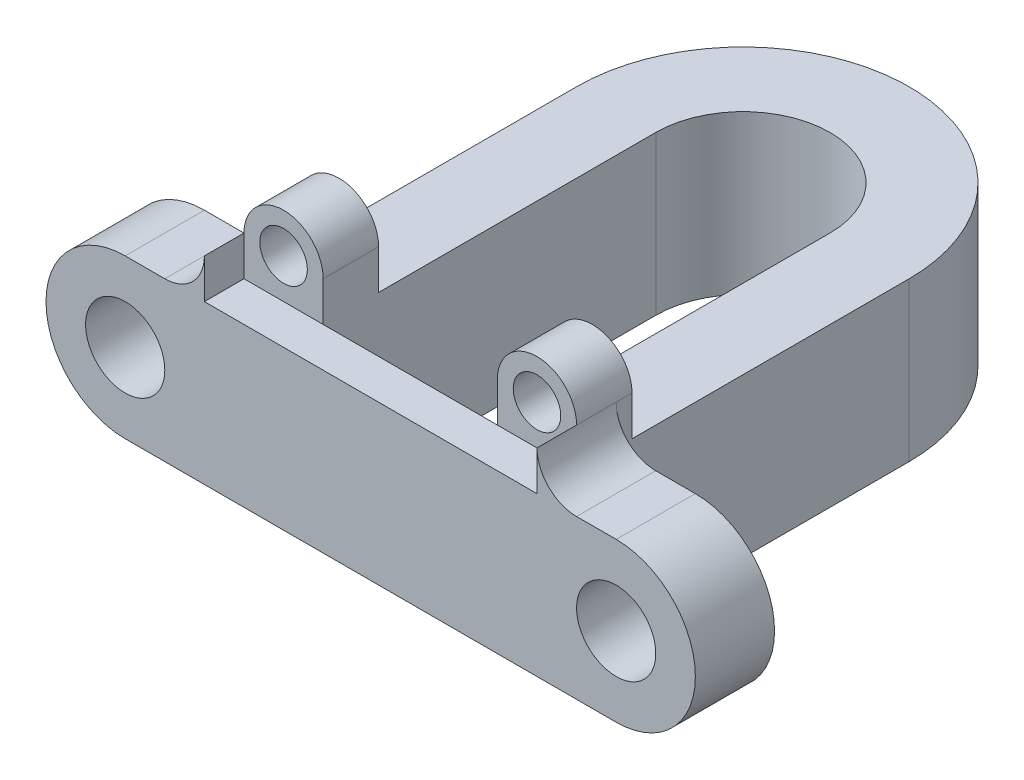
ISO-10303-21;
HEADER;
FILE_DESCRIPTION(('STEP AP214'),'2;1');
FILE_NAME('part.step','',(''),(''),'','','');
FILE_SCHEMA(('AUTOMOTIVE_DESIGN { 1 0 10303 214 1 1 1 1 }'));
ENDSEC;
DATA;
#1=APPLICATION_CONTEXT('core data for automotive mechanical design processes');
#2=APPLICATION_PROTOCOL_DEFINITION('international standard','automotive_design',2000,#1);
#3=PRODUCT_CONTEXT('',#1,'mechanical');
#4=PRODUCT('Part','Part','',(#3));
#5=PRODUCT_RELATED_PRODUCT_CATEGORY('part','',(#4));
#6=PRODUCT_DEFINITION_FORMATION('','',#4);
#7=PRODUCT_DEFINITION_CONTEXT('part definition',#1,'design');
#8=PRODUCT_DEFINITION('design','',#6,#7);
#9=PRODUCT_DEFINITION_SHAPE('','',#8);
#10=(LENGTH_UNIT() NAMED_UNIT(*) SI_UNIT(.MILLI.,.METRE.));
#11=(NAMED_UNIT(*) PLANE_ANGLE_UNIT() SI_UNIT($,.RADIAN.));
#12=(NAMED_UNIT(*) SI_UNIT($,.STERADIAN.) SOLID_ANGLE_UNIT());
#13=UNCERTAINTY_MEASURE_WITH_UNIT(LENGTH_MEASURE(1.E-05),#10,'distance_accuracy_value','');
#14=(GEOMETRIC_REPRESENTATION_CONTEXT(3) GLOBAL_UNCERTAINTY_ASSIGNED_CONTEXT((#13)) GLOBAL_UNIT_ASSIGNED_CONTEXT((#10,
#11,#12)) REPRESENTATION_CONTEXT('',''));
#15=CARTESIAN_POINT('',(0.,0.,0.));
#16=DIRECTION('',(0.,0.,1.));
#17=DIRECTION('',(1.,0.,0.));
#18=AXIS2_PLACEMENT_3D('',#15,#16,#17);
#19=CARTESIAN_POINT('',(42.,0.,5.));
#20=DIRECTION('',(-1.,0.,0.));
#21=DIRECTION('',(0.,0.,1.));
#22=AXIS2_PLACEMENT_3D('',#19,#20,#21);
#23=PLANE('',#22);
#24=DIRECTION('',(0.,1.,0.));
#25=VECTOR('',#24,1.);
#26=CARTESIAN_POINT('',(42.,20.,-5.));
#27=LINE('',#26,#25);
#28=CARTESIAN_POINT('',(42.,0.,-5.));
#29=VERTEX_POINT('',#28);
#30=CARTESIAN_POINT('',(42.,25.,-5.));
#31=VERTEX_POINT('',#30);
#32=EDGE_CURVE('E53',#29,#31,#27,.T.);
#33=ORIENTED_EDGE('',*,*,#32,.F.);
#34=DIRECTION('',(0.,0.,-1.));
#35=VECTOR('',#34,1.);
#36=CARTESIAN_POINT('',(42.,0.,5.));
#37=LINE('',#36,#35);
#38=CARTESIAN_POINT('',(42.,0.,-42.));
#39=VERTEX_POINT('',#38);
#40=EDGE_CURVE('E50',#29,#39,#37,.T.);
#41=ORIENTED_EDGE('',*,*,#40,.T.);
#42=DIRECTION('',(0.,1.,0.));
#43=VECTOR('',#42,1.);
#44=CARTESIAN_POINT('',(42.,0.,-42.));
#45=LINE('',#44,#43);
#46=CARTESIAN_POINT('',(42.,20.,-42.));
#47=VERTEX_POINT('',#46);
#48=EDGE_CURVE('E386',#39,#47,#45,.T.);
#49=ORIENTED_EDGE('',*,*,#48,.T.);
#50=DIRECTION('',(0.,0.,-1.));
#51=VECTOR('',#50,1.);
#52=CARTESIAN_POINT('',(42.,20.,5.));
#53=LINE('',#52,#51);
#54=CARTESIAN_POINT('',(42.,20.,-7.));
#55=VERTEX_POINT('',#54);
#56=EDGE_CURVE('E398',#55,#47,#53,.T.);
#57=ORIENTED_EDGE('',*,*,#56,.F.);
#58=DIRECTION('',(0.,-1.,0.));
#59=VECTOR('',#58,1.);
#60=CARTESIAN_POINT('',(42.,25.,-7.));
#61=LINE('',#60,#59);
#62=CARTESIAN_POINT('',(42.,25.,-7.));
#63=VERTEX_POINT('',#62);
#64=EDGE_CURVE('E291',#63,#55,#61,.T.);
#65=ORIENTED_EDGE('',*,*,#64,.F.);
#66=DIRECTION('',(0.,0.,1.));
#67=VECTOR('',#66,1.);
#68=CARTESIAN_POINT('',(42.,25.,-7.));
#69=LINE('',#68,#67);
#70=EDGE_CURVE('E315',#63,#31,#69,.T.);
#71=ORIENTED_EDGE('',*,*,#70,.T.);
#72=EDGE_LOOP('',(#33,#41,#49,#57,#65,#71));
#73=FACE_BOUND('',#72,.T.);
#74=ADVANCED_FACE('F39',(#73),#23,.F.);
#75=CARTESIAN_POINT('',(0.,20.,5.));
#76=DIRECTION('',(1.,0.,0.));
#77=DIRECTION('',(0.,0.,-1.));
#78=AXIS2_PLACEMENT_3D('',#75,#76,#77);
#79=PLANE('',#78);
#80=DIRECTION('',(0.,1.,0.));
#81=VECTOR('',#80,1.);
#82=CARTESIAN_POINT('',(0.,25.,-5.));
#83=LINE('',#82,#81);
#84=CARTESIAN_POINT('',(0.,0.,-5.));
#85=VERTEX_POINT('',#84);
#86=CARTESIAN_POINT('',(0.,25.,-5.));
#87=VERTEX_POINT('',#86);
#88=EDGE_CURVE('E267',#85,#87,#83,.T.);
#89=ORIENTED_EDGE('',*,*,#88,.T.);
#90=DIRECTION('',(0.,0.,1.));
#91=VECTOR('',#90,1.);
#92=CARTESIAN_POINT('',(0.,25.,-7.));
#93=LINE('',#92,#91);
#94=CARTESIAN_POINT('',(0.,25.,-7.));
#95=VERTEX_POINT('',#94);
#96=EDGE_CURVE('E341',#95,#87,#93,.T.);
#97=ORIENTED_EDGE('',*,*,#96,.F.);
#98=DIRECTION('',(0.,-1.,0.));
#99=VECTOR('',#98,1.);
#100=CARTESIAN_POINT('',(0.,25.,-7.));
#101=LINE('',#100,#99);
#102=CARTESIAN_POINT('',(0.,20.,-7.));
#103=VERTEX_POINT('',#102);
#104=EDGE_CURVE('E329',#95,#103,#101,.T.);
#105=ORIENTED_EDGE('',*,*,#104,.T.);
#106=DIRECTION('',(0.,0.,-1.));
#107=VECTOR('',#106,1.);
#108=CARTESIAN_POINT('',(0.,20.,5.));
#109=LINE('',#108,#107);
#110=CARTESIAN_POINT('',(0.,20.,-42.));
#111=VERTEX_POINT('',#110);
#112=EDGE_CURVE('E399',#103,#111,#109,.T.);
#113=ORIENTED_EDGE('',*,*,#112,.T.);
#114=DIRECTION('',(0.,1.,0.));
#115=VECTOR('',#114,1.);
#116=CARTESIAN_POINT('',(0.,0.,-42.));
#117=LINE('',#116,#115);
#118=CARTESIAN_POINT('',(0.,0.,-42.));
#119=VERTEX_POINT('',#118);
#120=EDGE_CURVE('E387',#119,#111,#117,.T.);
#121=ORIENTED_EDGE('',*,*,#120,.F.);
#122=DIRECTION('',(0.,0.,-1.));
#123=VECTOR('',#122,1.);
#124=CARTESIAN_POINT('',(0.,0.,5.));
#125=LINE('',#124,#123);
#126=EDGE_CURVE('E11',#85,#119,#125,.T.);
#127=ORIENTED_EDGE('',*,*,#126,.F.);
#128=EDGE_LOOP('',(#89,#97,#105,#113,#121,#127));
#129=FACE_BOUND('',#128,.T.);
#130=ADVANCED_FACE('F41',(#129),#79,.F.);
#131=CARTESIAN_POINT('',(42.,20.,5.));
#132=DIRECTION('',(0.,-1.,0.));
#133=DIRECTION('',(0.,0.,-1.));
#134=AXIS2_PLACEMENT_3D('',#131,#132,#133);
#135=PLANE('',#134);
#136=DIRECTION('',(-1.,0.,0.));
#137=VECTOR('',#136,1.);
#138=CARTESIAN_POINT('',(42.,20.,-7.));
#139=LINE('',#138,#137);
#140=CARTESIAN_POINT('',(32.,20.,-7.));
#141=VERTEX_POINT('',#140);
#142=EDGE_CURVE('E293',#55,#141,#139,.T.);
#143=ORIENTED_EDGE('',*,*,#142,.F.);
#144=ORIENTED_EDGE('',*,*,#56,.T.);
#145=CARTESIAN_POINT('',(21.,20.,-42.));
#146=DIRECTION('',(0.,1.,0.));
#147=DIRECTION('',(0.,0.,1.));
#148=AXIS2_PLACEMENT_3D('',#145,#146,#147);
#149=CIRCLE('',#148,21.);
#150=EDGE_CURVE('E372',#47,#111,#149,.T.);
#151=ORIENTED_EDGE('',*,*,#150,.T.);
#152=ORIENTED_EDGE('',*,*,#112,.F.);
#153=DIRECTION('',(1.,0.,0.));
#154=VECTOR('',#153,1.);
#155=CARTESIAN_POINT('',(0.,20.,-7.));
#156=LINE('',#155,#154);
#157=CARTESIAN_POINT('',(10.,20.,-7.00000000000001));
#158=VERTEX_POINT('',#157);
#159=EDGE_CURVE('E318',#103,#158,#156,.T.);
#160=ORIENTED_EDGE('',*,*,#159,.T.);
#161=DIRECTION('',(0.,0.,1.));
#162=VECTOR('',#161,1.);
#163=CARTESIAN_POINT('',(10.,20.,-42.));
#164=LINE('',#163,#162);
#165=CARTESIAN_POINT('',(10.,20.,-42.));
#166=VERTEX_POINT('',#165);
#167=EDGE_CURVE('E364',#166,#158,#164,.T.);
#168=ORIENTED_EDGE('',*,*,#167,.F.);
#169=CARTESIAN_POINT('',(21.,20.,-42.));
#170=DIRECTION('',(0.,1.,0.));
#171=DIRECTION('',(0.,0.,1.));
#172=AXIS2_PLACEMENT_3D('',#169,#170,#171);
#173=CIRCLE('',#172,11.);
#174=CARTESIAN_POINT('',(32.,20.,-42.));
#175=VERTEX_POINT('',#174);
#176=EDGE_CURVE('E350',#175,#166,#173,.T.);
#177=ORIENTED_EDGE('',*,*,#176,.F.);
#178=DIRECTION('',(0.,0.,-1.));
#179=VECTOR('',#178,1.);
#180=CARTESIAN_POINT('',(32.,20.,0.));
#181=LINE('',#180,#179);
#182=EDGE_CURVE('E355',#141,#175,#181,.T.);
#183=ORIENTED_EDGE('',*,*,#182,.F.);
#184=EDGE_LOOP('',(#143,#144,#151,#152,#160,#168,#177,#183));
#185=FACE_BOUND('',#184,.T.);
#186=ADVANCED_FACE('F420',(#185),#135,.F.);
#187=CARTESIAN_POINT('',(42.,20.,5.));
#188=VERTEX_POINT('',#187);
#189=CARTESIAN_POINT('',(42.,20.,0.));
#190=VERTEX_POINT('',#189);
#191=EDGE_CURVE('E402',#188,#190,#53,.T.);
#192=ORIENTED_EDGE('',*,*,#191,.T.);
#193=DIRECTION('',(-1.,0.,0.));
#194=VECTOR('',#193,1.);
#195=CARTESIAN_POINT('',(42.,20.,0.));
#196=LINE('',#195,#194);
#197=CARTESIAN_POINT('',(32.,20.,0.));
#198=VERTEX_POINT('',#197);
#199=EDGE_CURVE('E290',#190,#198,#196,.T.);
#200=ORIENTED_EDGE('',*,*,#199,.T.);
#201=DIRECTION('',(1.,0.,0.));
#202=VECTOR('',#201,1.);
#203=CARTESIAN_POINT('',(10.,20.,0.));
#204=LINE('',#203,#202);
#205=CARTESIAN_POINT('',(10.,20.,0.));
#206=VERTEX_POINT('',#205);
#207=EDGE_CURVE('E370',#206,#198,#204,.T.);
#208=ORIENTED_EDGE('',*,*,#207,.F.);
#209=DIRECTION('',(1.,0.,0.));
#210=VECTOR('',#209,1.);
#211=CARTESIAN_POINT('',(0.,20.,0.));
#212=LINE('',#211,#210);
#213=CARTESIAN_POINT('',(0.,20.,0.));
#214=VERTEX_POINT('',#213);
#215=EDGE_CURVE('E320',#214,#206,#212,.T.);
#216=ORIENTED_EDGE('',*,*,#215,.F.);
#217=CARTESIAN_POINT('',(0.,20.,5.));
#218=VERTEX_POINT('',#217);
#219=EDGE_CURVE('E400',#218,#214,#109,.T.);
#220=ORIENTED_EDGE('',*,*,#219,.F.);
#221=DIRECTION('',(-1.,0.,0.));
#222=VECTOR('',#221,1.);
#223=CARTESIAN_POINT('',(42.,20.,5.));
#224=LINE('',#223,#222);
#225=EDGE_CURVE('E394',#188,#218,#224,.T.);
#226=ORIENTED_EDGE('',*,*,#225,.F.);
#227=EDGE_LOOP('',(#192,#200,#208,#216,#220,#226));
#228=FACE_BOUND('',#227,.T.);
#229=ADVANCED_FACE('F455',(#228),#135,.F.);
#230=CARTESIAN_POINT('',(0.,0.,5.));
#231=DIRECTION('',(0.,1.,0.));
#232=DIRECTION('',(0.,0.,1.));
#233=AXIS2_PLACEMENT_3D('',#230,#231,#232);
#234=PLANE('',#233);
#235=DIRECTION('',(0.,0.,-1.));
#236=VECTOR('',#235,1.);
#237=CARTESIAN_POINT('',(32.,0.,0.));
#238=LINE('',#237,#236);
#239=CARTESIAN_POINT('',(32.,0.,0.));
#240=VERTEX_POINT('',#239);
#241=CARTESIAN_POINT('',(32.,0.,-42.));
#242=VERTEX_POINT('',#241);
#243=EDGE_CURVE('E360',#240,#242,#238,.T.);
#244=ORIENTED_EDGE('',*,*,#243,.T.);
#245=CARTESIAN_POINT('',(21.,0.,-42.));
#246=DIRECTION('',(0.,1.,0.));
#247=DIRECTION('',(0.,0.,1.));
#248=AXIS2_PLACEMENT_3D('',#245,#246,#247);
#249=CIRCLE('',#248,11.);
#250=CARTESIAN_POINT('',(10.,0.,-42.));
#251=VERTEX_POINT('',#250);
#252=EDGE_CURVE('E347',#242,#251,#249,.T.);
#253=ORIENTED_EDGE('',*,*,#252,.T.);
#254=DIRECTION('',(0.,0.,1.));
#255=VECTOR('',#254,1.);
#256=CARTESIAN_POINT('',(10.,0.,-42.));
#257=LINE('',#256,#255);
#258=CARTESIAN_POINT('',(10.,0.,0.));
#259=VERTEX_POINT('',#258);
#260=EDGE_CURVE('E354',#251,#259,#257,.T.);
#261=ORIENTED_EDGE('',*,*,#260,.T.);
#262=DIRECTION('',(1.,0.,0.));
#263=VECTOR('',#262,1.);
#264=CARTESIAN_POINT('',(10.,0.,0.));
#265=LINE('',#264,#263);
#266=EDGE_CURVE('E358',#259,#240,#265,.T.);
#267=ORIENTED_EDGE('',*,*,#266,.T.);
#268=EDGE_LOOP('',(#244,#253,#261,#267));
#269=FACE_BOUND('',#268,.T.);
#270=DIRECTION('',(1.,0.,0.));
#271=VECTOR('',#270,1.);
#272=CARTESIAN_POINT('',(0.,0.,5.));
#273=LINE('',#272,#271);
#274=CARTESIAN_POINT('',(-10.,0.,5.));
#275=VERTEX_POINT('',#274);
#276=CARTESIAN_POINT('',(52.,0.,5.));
#277=VERTEX_POINT('',#276);
#278=EDGE_CURVE('E220',#275,#277,#273,.T.);
#279=ORIENTED_EDGE('',*,*,#278,.F.);
#280=DIRECTION('',(0.,0.,-1.));
#281=VECTOR('',#280,1.);
#282=CARTESIAN_POINT('',(-10.,0.,5.));
#283=LINE('',#282,#281);
#284=CARTESIAN_POINT('',(-10.,0.,-5.));
#285=VERTEX_POINT('',#284);
#286=EDGE_CURVE('E283',#275,#285,#283,.T.);
#287=ORIENTED_EDGE('',*,*,#286,.T.);
#288=DIRECTION('',(1.,0.,0.));
#289=VECTOR('',#288,1.);
#290=CARTESIAN_POINT('',(0.,0.,-5.));
#291=LINE('',#290,#289);
#292=EDGE_CURVE('E261',#285,#85,#291,.T.);
#293=ORIENTED_EDGE('',*,*,#292,.T.);
#294=ORIENTED_EDGE('',*,*,#126,.T.);
#295=CARTESIAN_POINT('',(21.,0.,-42.));
#296=DIRECTION('',(0.,1.,0.));
#297=DIRECTION('',(0.,0.,1.));
#298=AXIS2_PLACEMENT_3D('',#295,#296,#297);
#299=CIRCLE('',#298,21.);
#300=EDGE_CURVE('E384',#39,#119,#299,.T.);
#301=ORIENTED_EDGE('',*,*,#300,.F.);
#302=ORIENTED_EDGE('',*,*,#40,.F.);
#303=DIRECTION('',(-1.,0.,0.));
#304=VECTOR('',#303,1.);
#305=CARTESIAN_POINT('',(42.,0.,-5.));
#306=LINE('',#305,#304);
#307=CARTESIAN_POINT('',(52.,0.,-5.));
#308=VERTEX_POINT('',#307);
#309=EDGE_CURVE('E217',#308,#29,#306,.T.);
#310=ORIENTED_EDGE('',*,*,#309,.F.);
#311=DIRECTION('',(0.,0.,-1.));
#312=VECTOR('',#311,1.);
#313=CARTESIAN_POINT('',(52.,0.,5.));
#314=LINE('',#313,#312);
#315=EDGE_CURVE('E230',#277,#308,#314,.T.);
#316=ORIENTED_EDGE('',*,*,#315,.F.);
#317=EDGE_LOOP('',(#279,#287,#293,#294,#301,#302,#310,#316));
#318=FACE_BOUND('',#317,.T.);
#319=ADVANCED_FACE('F413',(#269,#318),#234,.F.);
#320=CARTESIAN_POINT('',(0.,0.,5.));
#321=DIRECTION('',(0.,0.,1.));
#322=DIRECTION('',(1.,0.,0.));
#323=AXIS2_PLACEMENT_3D('',#320,#321,#322);
#324=PLANE('',#323);
#325=ORIENTED_EDGE('',*,*,#225,.T.);
#326=DIRECTION('',(0.,1.,0.));
#327=VECTOR('',#326,1.);
#328=CARTESIAN_POINT('',(0.,20.,5.));
#329=LINE('',#328,#327);
#330=CARTESIAN_POINT('',(0.,25.,5.));
#331=VERTEX_POINT('',#330);
#332=EDGE_CURVE('E254',#218,#331,#329,.T.);
#333=ORIENTED_EDGE('',*,*,#332,.T.);
#334=CARTESIAN_POINT('',(-5.,25.,5.));
#335=DIRECTION('',(0.,0.,-1.));
#336=DIRECTION('',(1.,0.,0.));
#337=AXIS2_PLACEMENT_3D('',#334,#335,#336);
#338=CIRCLE('',#337,5.00000000000001);
#339=CARTESIAN_POINT('',(-5.,20.,5.));
#340=VERTEX_POINT('',#339);
#341=EDGE_CURVE('E257',#331,#340,#338,.T.);
#342=ORIENTED_EDGE('',*,*,#341,.T.);
#343=DIRECTION('',(-1.,0.,0.));
#344=VECTOR('',#343,1.);
#345=CARTESIAN_POINT('',(-10.,20.,5.));
#346=LINE('',#345,#344);
#347=CARTESIAN_POINT('',(-10.,20.,5.));
#348=VERTEX_POINT('',#347);
#349=EDGE_CURVE('E259',#340,#348,#346,.T.);
#350=ORIENTED_EDGE('',*,*,#349,.T.);
#351=CARTESIAN_POINT('',(-10.,10.,5.));
#352=DIRECTION('',(0.,0.,1.));
#353=DIRECTION('',(1.,0.,0.));
#354=AXIS2_PLACEMENT_3D('',#351,#352,#353);
#355=CIRCLE('',#354,10.);
#356=EDGE_CURVE('E252',#348,#275,#355,.T.);
#357=ORIENTED_EDGE('',*,*,#356,.T.);
#358=ORIENTED_EDGE('',*,*,#278,.T.);
#359=CARTESIAN_POINT('',(52.,10.,5.));
#360=DIRECTION('',(0.,0.,-1.));
#361=DIRECTION('',(-1.,0.,0.));
#362=AXIS2_PLACEMENT_3D('',#359,#360,#361);
#363=CIRCLE('',#362,10.);
#364=CARTESIAN_POINT('',(52.,20.,5.));
#365=VERTEX_POINT('',#364);
#366=EDGE_CURVE('E196',#365,#277,#363,.T.);
#367=ORIENTED_EDGE('',*,*,#366,.F.);
#368=DIRECTION('',(1.,0.,0.));
#369=VECTOR('',#368,1.);
#370=CARTESIAN_POINT('',(52.,20.,5.));
#371=LINE('',#370,#369);
#372=CARTESIAN_POINT('',(47.,20.,5.));
#373=VERTEX_POINT('',#372);
#374=EDGE_CURVE('E211',#373,#365,#371,.T.);
#375=ORIENTED_EDGE('',*,*,#374,.F.);
#376=CARTESIAN_POINT('',(47.,25.,5.));
#377=DIRECTION('',(0.,0.,1.));
#378=DIRECTION('',(-1.,0.,0.));
#379=AXIS2_PLACEMENT_3D('',#376,#377,#378);
#380=CIRCLE('',#379,5.00000000000001);
#381=CARTESIAN_POINT('',(42.,25.,5.));
#382=VERTEX_POINT('',#381);
#383=EDGE_CURVE('E224',#382,#373,#380,.T.);
#384=ORIENTED_EDGE('',*,*,#383,.F.);
#385=DIRECTION('',(0.,1.,0.));
#386=VECTOR('',#385,1.);
#387=CARTESIAN_POINT('',(42.,25.,5.));
#388=LINE('',#387,#386);
#389=EDGE_CURVE('E221',#188,#382,#388,.T.);
#390=ORIENTED_EDGE('',*,*,#389,.F.);
#391=EDGE_LOOP('',(#325,#333,#342,#350,#357,#358,#367,#375,#384,#390));
#392=FACE_BOUND('',#391,.T.);
#393=CARTESIAN_POINT('',(-10.,10.,5.));
#394=DIRECTION('',(0.,0.,1.));
#395=DIRECTION('',(1.,0.,0.));
#396=AXIS2_PLACEMENT_3D('',#393,#394,#395);
#397=CIRCLE('',#396,5.);
#398=CARTESIAN_POINT('',(-5.,10.,5.));
#399=VERTEX_POINT('',#398);
#400=EDGE_CURVE('E244',#399,#399,#397,.T.);
#401=ORIENTED_EDGE('',*,*,#400,.F.);
#402=EDGE_LOOP('',(#401));
#403=FACE_BOUND('',#402,.T.);
#404=CARTESIAN_POINT('',(52.,10.,5.));
#405=DIRECTION('',(0.,0.,-1.));
#406=DIRECTION('',(-1.,0.,0.));
#407=AXIS2_PLACEMENT_3D('',#404,#405,#406);
#408=CIRCLE('',#407,5.);
#409=CARTESIAN_POINT('',(47.,10.,5.));
#410=VERTEX_POINT('',#409);
#411=EDGE_CURVE('E235',#410,#410,#408,.T.);
#412=ORIENTED_EDGE('',*,*,#411,.T.);
#413=EDGE_LOOP('',(#412));
#414=FACE_BOUND('',#413,.T.);
#415=ADVANCED_FACE('F212',(#392,#403,#414),#324,.T.);
#416=CARTESIAN_POINT('',(21.,0.,-42.));
#417=DIRECTION('',(0.,1.,0.));
#418=DIRECTION('',(0.,0.,1.));
#419=AXIS2_PLACEMENT_3D('',#416,#417,#418);
#420=CYLINDRICAL_SURFACE('',#419,21.);
#421=ORIENTED_EDGE('',*,*,#150,.F.);
#422=ORIENTED_EDGE('',*,*,#48,.F.);
#423=ORIENTED_EDGE('',*,*,#300,.T.);
#424=ORIENTED_EDGE('',*,*,#120,.T.);
#425=EDGE_LOOP('',(#421,#422,#423,#424));
#426=FACE_BOUND('',#425,.T.);
#427=ADVANCED_FACE('F408',(#426),#420,.T.);
#428=CARTESIAN_POINT('',(21.,0.,-42.));
#429=DIRECTION('',(0.,1.,0.));
#430=DIRECTION('',(0.,0.,1.));
#431=AXIS2_PLACEMENT_3D('',#428,#429,#430);
#432=CYLINDRICAL_SURFACE('',#431,11.);
#433=ORIENTED_EDGE('',*,*,#176,.T.);
#434=DIRECTION('',(0.,1.,0.));
#435=VECTOR('',#434,1.);
#436=CARTESIAN_POINT('',(10.,0.,-42.));
#437=LINE('',#436,#435);
#438=EDGE_CURVE('E365',#251,#166,#437,.T.);
#439=ORIENTED_EDGE('',*,*,#438,.F.);
#440=ORIENTED_EDGE('',*,*,#252,.F.);
#441=DIRECTION('',(0.,1.,0.));
#442=VECTOR('',#441,1.);
#443=CARTESIAN_POINT('',(32.,0.,-42.));
#444=LINE('',#443,#442);
#445=EDGE_CURVE('E371',#242,#175,#444,.T.);
#446=ORIENTED_EDGE('',*,*,#445,.T.);
#447=EDGE_LOOP('',(#433,#439,#440,#446));
#448=FACE_BOUND('',#447,.T.);
#449=ADVANCED_FACE('F467',(#448),#432,.F.);
#450=CARTESIAN_POINT('',(32.,0.,0.));
#451=DIRECTION('',(1.,0.,0.));
#452=DIRECTION('',(0.,0.,-1.));
#453=AXIS2_PLACEMENT_3D('',#450,#451,#452);
#454=PLANE('',#453);
#455=DIRECTION('',(0.,1.,0.));
#456=VECTOR('',#455,1.);
#457=CARTESIAN_POINT('',(32.,0.,0.));
#458=LINE('',#457,#456);
#459=EDGE_CURVE('E374',#240,#198,#458,.T.);
#460=ORIENTED_EDGE('',*,*,#459,.T.);
#461=DIRECTION('',(0.,1.,0.));
#462=VECTOR('',#461,1.);
#463=CARTESIAN_POINT('',(32.,20.,0.));
#464=LINE('',#463,#462);
#465=CARTESIAN_POINT('',(32.,25.,0.));
#466=VERTEX_POINT('',#465);
#467=EDGE_CURVE('E295',#198,#466,#464,.T.);
#468=ORIENTED_EDGE('',*,*,#467,.T.);
#469=DIRECTION('',(0.,0.,1.));
#470=VECTOR('',#469,1.);
#471=CARTESIAN_POINT('',(32.,25.,-7.));
#472=LINE('',#471,#470);
#473=CARTESIAN_POINT('',(32.,25.,-7.));
#474=VERTEX_POINT('',#473);
#475=EDGE_CURVE('E308',#474,#466,#472,.T.);
#476=ORIENTED_EDGE('',*,*,#475,.F.);
#477=DIRECTION('',(0.,1.,0.));
#478=VECTOR('',#477,1.);
#479=CARTESIAN_POINT('',(32.,20.,-7.));
#480=LINE('',#479,#478);
#481=EDGE_CURVE('E296',#141,#474,#480,.T.);
#482=ORIENTED_EDGE('',*,*,#481,.F.);
#483=ORIENTED_EDGE('',*,*,#182,.T.);
#484=ORIENTED_EDGE('',*,*,#445,.F.);
#485=ORIENTED_EDGE('',*,*,#243,.F.);
#486=EDGE_LOOP('',(#460,#468,#476,#482,#483,#484,#485));
#487=FACE_BOUND('',#486,.T.);
#488=ADVANCED_FACE('F465',(#487),#454,.F.);
#489=CARTESIAN_POINT('',(10.,0.,0.));
#490=DIRECTION('',(0.,0.,1.));
#491=DIRECTION('',(1.,0.,0.));
#492=AXIS2_PLACEMENT_3D('',#489,#490,#491);
#493=PLANE('',#492);
#494=ORIENTED_EDGE('',*,*,#207,.T.);
#495=ORIENTED_EDGE('',*,*,#459,.F.);
#496=ORIENTED_EDGE('',*,*,#266,.F.);
#497=DIRECTION('',(0.,1.,0.));
#498=VECTOR('',#497,1.);
#499=CARTESIAN_POINT('',(10.,0.,0.));
#500=LINE('',#499,#498);
#501=EDGE_CURVE('E377',#259,#206,#500,.T.);
#502=ORIENTED_EDGE('',*,*,#501,.T.);
#503=EDGE_LOOP('',(#494,#495,#496,#502));
#504=FACE_BOUND('',#503,.T.);
#505=ADVANCED_FACE('F471',(#504),#493,.F.);
#506=CARTESIAN_POINT('',(10.,0.,-42.));
#507=DIRECTION('',(-1.,0.,0.));
#508=DIRECTION('',(0.,0.,1.));
#509=AXIS2_PLACEMENT_3D('',#506,#507,#508);
#510=PLANE('',#509);
#511=ORIENTED_EDGE('',*,*,#167,.T.);
#512=DIRECTION('',(0.,1.,0.));
#513=VECTOR('',#512,1.);
#514=CARTESIAN_POINT('',(10.,20.,-7.));
#515=LINE('',#514,#513);
#516=CARTESIAN_POINT('',(10.,25.,-7.));
#517=VERTEX_POINT('',#516);
#518=EDGE_CURVE('E324',#158,#517,#515,.T.);
#519=ORIENTED_EDGE('',*,*,#518,.T.);
#520=DIRECTION('',(0.,0.,1.));
#521=VECTOR('',#520,1.);
#522=CARTESIAN_POINT('',(10.,25.,-7.));
#523=LINE('',#522,#521);
#524=CARTESIAN_POINT('',(10.,25.,0.));
#525=VERTEX_POINT('',#524);
#526=EDGE_CURVE('E335',#517,#525,#523,.T.);
#527=ORIENTED_EDGE('',*,*,#526,.T.);
#528=DIRECTION('',(0.,1.,0.));
#529=VECTOR('',#528,1.);
#530=CARTESIAN_POINT('',(10.,20.,0.));
#531=LINE('',#530,#529);
#532=EDGE_CURVE('E337',#206,#525,#531,.T.);
#533=ORIENTED_EDGE('',*,*,#532,.F.);
#534=ORIENTED_EDGE('',*,*,#501,.F.);
#535=ORIENTED_EDGE('',*,*,#260,.F.);
#536=ORIENTED_EDGE('',*,*,#438,.T.);
#537=EDGE_LOOP('',(#511,#519,#527,#533,#534,#535,#536));
#538=FACE_BOUND('',#537,.T.);
#539=ADVANCED_FACE('F472',(#538),#510,.F.);
#540=CARTESIAN_POINT('',(5.00000000000001,25.,-7.));
#541=DIRECTION('',(0.,0.,1.));
#542=DIRECTION('',(1.,0.,0.));
#543=AXIS2_PLACEMENT_3D('',#540,#541,#542);
#544=CYLINDRICAL_SURFACE('',#543,5.);
#545=CARTESIAN_POINT('',(5.00000000000001,25.,0.));
#546=DIRECTION('',(0.,0.,1.));
#547=DIRECTION('',(1.,0.,0.));
#548=AXIS2_PLACEMENT_3D('',#545,#546,#547);
#549=CIRCLE('',#548,5.);
#550=CARTESIAN_POINT('',(0.,25.,0.));
#551=VERTEX_POINT('',#550);
#552=EDGE_CURVE('E339',#525,#551,#549,.T.);
#553=ORIENTED_EDGE('',*,*,#552,.F.);
#554=ORIENTED_EDGE('',*,*,#526,.F.);
#555=CARTESIAN_POINT('',(5.00000000000001,25.,-7.));
#556=DIRECTION('',(0.,0.,1.));
#557=DIRECTION('',(1.,0.,0.));
#558=AXIS2_PLACEMENT_3D('',#555,#556,#557);
#559=CIRCLE('',#558,5.);
#560=EDGE_CURVE('E330',#517,#95,#559,.T.);
#561=ORIENTED_EDGE('',*,*,#560,.T.);
#562=ORIENTED_EDGE('',*,*,#96,.T.);
#563=DIRECTION('',(0.,0.,-1.));
#564=VECTOR('',#563,1.);
#565=CARTESIAN_POINT('',(0.,25.,5.));
#566=LINE('',#565,#564);
#567=EDGE_CURVE('E280',#551,#87,#566,.T.);
#568=ORIENTED_EDGE('',*,*,#567,.F.);
#569=EDGE_LOOP('',(#553,#554,#561,#562,#568));
#570=FACE_BOUND('',#569,.T.);
#571=ADVANCED_FACE('F483',(#570),#544,.T.);
#572=CARTESIAN_POINT('',(5.00000000000001,25.,-7.));
#573=DIRECTION('',(0.,0.,1.));
#574=DIRECTION('',(1.,0.,0.));
#575=AXIS2_PLACEMENT_3D('',#572,#573,#574);
#576=PLANE('',#575);
#577=CARTESIAN_POINT('',(5.00000000000001,25.,-7.));
#578=DIRECTION('',(0.,0.,1.));
#579=DIRECTION('',(1.,0.,0.));
#580=AXIS2_PLACEMENT_3D('',#577,#578,#579);
#581=CIRCLE('',#580,3.);
#582=CARTESIAN_POINT('',(8.00000000000001,25.,-7.));
#583=VERTEX_POINT('',#582);
#584=EDGE_CURVE('E313',#583,#583,#581,.T.);
#585=ORIENTED_EDGE('',*,*,#584,.T.);
#586=EDGE_LOOP('',(#585));
#587=FACE_BOUND('',#586,.T.);
#588=ORIENTED_EDGE('',*,*,#159,.F.);
#589=ORIENTED_EDGE('',*,*,#104,.F.);
#590=ORIENTED_EDGE('',*,*,#560,.F.);
#591=ORIENTED_EDGE('',*,*,#518,.F.);
#592=EDGE_LOOP('',(#588,#589,#590,#591));
#593=FACE_BOUND('',#592,.T.);
#594=ADVANCED_FACE('F484',(#587,#593),#576,.F.);
#595=CARTESIAN_POINT('',(5.00000000000001,25.,0.));
#596=DIRECTION('',(0.,0.,1.));
#597=DIRECTION('',(1.,0.,0.));
#598=AXIS2_PLACEMENT_3D('',#595,#596,#597);
#599=PLANE('',#598);
#600=CARTESIAN_POINT('',(5.00000000000001,25.,0.));
#601=DIRECTION('',(0.,0.,1.));
#602=DIRECTION('',(1.,0.,0.));
#603=AXIS2_PLACEMENT_3D('',#600,#601,#602);
#604=CIRCLE('',#603,3.);
#605=CARTESIAN_POINT('',(8.00000000000001,25.,0.));
#606=VERTEX_POINT('',#605);
#607=EDGE_CURVE('E311',#606,#606,#604,.T.);
#608=ORIENTED_EDGE('',*,*,#607,.F.);
#609=EDGE_LOOP('',(#608));
#610=FACE_BOUND('',#609,.T.);
#611=ORIENTED_EDGE('',*,*,#215,.T.);
#612=ORIENTED_EDGE('',*,*,#532,.T.);
#613=ORIENTED_EDGE('',*,*,#552,.T.);
#614=DIRECTION('',(0.,-1.,0.));
#615=VECTOR('',#614,1.);
#616=CARTESIAN_POINT('',(0.,25.,0.));
#617=LINE('',#616,#615);
#618=EDGE_CURVE('E321',#551,#214,#617,.T.);
#619=ORIENTED_EDGE('',*,*,#618,.T.);
#620=EDGE_LOOP('',(#611,#612,#613,#619));
#621=FACE_BOUND('',#620,.T.);
#622=ADVANCED_FACE('F486',(#610,#621),#599,.T.);
#623=CARTESIAN_POINT('',(5.00000000000001,25.,-7.));
#624=DIRECTION('',(0.,0.,1.));
#625=DIRECTION('',(1.,0.,0.));
#626=AXIS2_PLACEMENT_3D('',#623,#624,#625);
#627=CYLINDRICAL_SURFACE('',#626,3.);
#628=ORIENTED_EDGE('',*,*,#584,.F.);
#629=EDGE_LOOP('',(#628));
#630=FACE_BOUND('',#629,.T.);
#631=ORIENTED_EDGE('',*,*,#607,.T.);
#632=EDGE_LOOP('',(#631));
#633=FACE_BOUND('',#632,.T.);
#634=ADVANCED_FACE('F534',(#630,#633),#627,.F.);
#635=CARTESIAN_POINT('',(37.,25.,-7.));
#636=DIRECTION('',(0.,0.,1.));
#637=DIRECTION('',(-1.,0.,0.));
#638=AXIS2_PLACEMENT_3D('',#635,#636,#637);
#639=PLANE('',#638);
#640=ORIENTED_EDGE('',*,*,#142,.T.);
#641=ORIENTED_EDGE('',*,*,#481,.T.);
#642=CARTESIAN_POINT('',(37.,25.,-7.));
#643=DIRECTION('',(0.,0.,-1.));
#644=DIRECTION('',(-1.,0.,0.));
#645=AXIS2_PLACEMENT_3D('',#642,#643,#644);
#646=CIRCLE('',#645,5.);
#647=EDGE_CURVE('E298',#474,#63,#646,.T.);
#648=ORIENTED_EDGE('',*,*,#647,.T.);
#649=ORIENTED_EDGE('',*,*,#64,.T.);
#650=EDGE_LOOP('',(#640,#641,#648,#649));
#651=FACE_BOUND('',#650,.T.);
#652=CARTESIAN_POINT('',(37.,25.,-7.));
#653=DIRECTION('',(0.,0.,-1.));
#654=DIRECTION('',(-1.,0.,0.));
#655=AXIS2_PLACEMENT_3D('',#652,#653,#654);
#656=CIRCLE('',#655,3.);
#657=CARTESIAN_POINT('',(34.,25.,-7.));
#658=VERTEX_POINT('',#657);
#659=EDGE_CURVE('E284',#658,#658,#656,.T.);
#660=ORIENTED_EDGE('',*,*,#659,.F.);
#661=EDGE_LOOP('',(#660));
#662=FACE_BOUND('',#661,.T.);
#663=ADVANCED_FACE('F422',(#651,#662),#639,.F.);
#664=CARTESIAN_POINT('',(37.,25.,0.));
#665=DIRECTION('',(0.,0.,1.));
#666=DIRECTION('',(-1.,0.,0.));
#667=AXIS2_PLACEMENT_3D('',#664,#665,#666);
#668=PLANE('',#667);
#669=ORIENTED_EDGE('',*,*,#199,.F.);
#670=DIRECTION('',(0.,-1.,0.));
#671=VECTOR('',#670,1.);
#672=CARTESIAN_POINT('',(42.,25.,0.));
#673=LINE('',#672,#671);
#674=CARTESIAN_POINT('',(42.,25.,0.));
#675=VERTEX_POINT('',#674);
#676=EDGE_CURVE('E305',#675,#190,#673,.T.);
#677=ORIENTED_EDGE('',*,*,#676,.F.);
#678=CARTESIAN_POINT('',(37.,25.,0.));
#679=DIRECTION('',(0.,0.,-1.));
#680=DIRECTION('',(-1.,0.,0.));
#681=AXIS2_PLACEMENT_3D('',#678,#679,#680);
#682=CIRCLE('',#681,5.);
#683=EDGE_CURVE('E304',#466,#675,#682,.T.);
#684=ORIENTED_EDGE('',*,*,#683,.F.);
#685=ORIENTED_EDGE('',*,*,#467,.F.);
#686=EDGE_LOOP('',(#669,#677,#684,#685));
#687=FACE_BOUND('',#686,.T.);
#688=CARTESIAN_POINT('',(37.,25.,0.));
#689=DIRECTION('',(0.,0.,-1.));
#690=DIRECTION('',(-1.,0.,0.));
#691=AXIS2_PLACEMENT_3D('',#688,#689,#690);
#692=CIRCLE('',#691,3.);
#693=CARTESIAN_POINT('',(34.,25.,0.));
#694=VERTEX_POINT('',#693);
#695=EDGE_CURVE('E282',#694,#694,#692,.T.);
#696=ORIENTED_EDGE('',*,*,#695,.T.);
#697=EDGE_LOOP('',(#696));
#698=FACE_BOUND('',#697,.T.);
#699=ADVANCED_FACE('F431',(#687,#698),#668,.T.);
#700=CARTESIAN_POINT('',(37.,25.,-7.));
#701=DIRECTION('',(0.,0.,1.));
#702=DIRECTION('',(1.,0.,0.));
#703=AXIS2_PLACEMENT_3D('',#700,#701,#702);
#704=CYLINDRICAL_SURFACE('',#703,5.);
#705=ORIENTED_EDGE('',*,*,#683,.T.);
#706=EDGE_CURVE('E65',#31,#675,#69,.T.);
#707=ORIENTED_EDGE('',*,*,#706,.F.);
#708=ORIENTED_EDGE('',*,*,#70,.F.);
#709=ORIENTED_EDGE('',*,*,#647,.F.);
#710=ORIENTED_EDGE('',*,*,#475,.T.);
#711=EDGE_LOOP('',(#705,#707,#708,#709,#710));
#712=FACE_BOUND('',#711,.T.);
#713=ADVANCED_FACE('F430',(#712),#704,.T.);
#714=CARTESIAN_POINT('',(37.,25.,-7.));
#715=DIRECTION('',(0.,0.,1.));
#716=DIRECTION('',(1.,0.,0.));
#717=AXIS2_PLACEMENT_3D('',#714,#715,#716);
#718=CYLINDRICAL_SURFACE('',#717,3.);
#719=ORIENTED_EDGE('',*,*,#659,.T.);
#720=EDGE_LOOP('',(#719));
#721=FACE_BOUND('',#720,.T.);
#722=ORIENTED_EDGE('',*,*,#695,.F.);
#723=EDGE_LOOP('',(#722));
#724=FACE_BOUND('',#723,.T.);
#725=ADVANCED_FACE('F427',(#721,#724),#718,.F.);
#726=CARTESIAN_POINT('',(0.,25.,5.));
#727=DIRECTION('',(-1.,0.,0.));
#728=DIRECTION('',(0.,-1.,0.));
#729=AXIS2_PLACEMENT_3D('',#726,#727,#728);
#730=PLANE('',#729);
#731=ORIENTED_EDGE('',*,*,#332,.F.);
#732=ORIENTED_EDGE('',*,*,#219,.T.);
#733=ORIENTED_EDGE('',*,*,#618,.F.);
#734=EDGE_CURVE('E279',#331,#551,#566,.T.);
#735=ORIENTED_EDGE('',*,*,#734,.F.);
#736=EDGE_LOOP('',(#731,#732,#733,#735));
#737=FACE_BOUND('',#736,.T.);
#738=ADVANCED_FACE('F438',(#737),#730,.F.);
#739=CARTESIAN_POINT('',(-10.,10.,-5.));
#740=DIRECTION('',(0.,0.,1.));
#741=DIRECTION('',(1.,0.,0.));
#742=AXIS2_PLACEMENT_3D('',#739,#740,#741);
#743=PLANE('',#742);
#744=CARTESIAN_POINT('',(-10.,10.,-5.));
#745=DIRECTION('',(0.,0.,1.));
#746=DIRECTION('',(1.,0.,0.));
#747=AXIS2_PLACEMENT_3D('',#744,#745,#746);
#748=CIRCLE('',#747,10.);
#749=CARTESIAN_POINT('',(-10.,20.,-5.));
#750=VERTEX_POINT('',#749);
#751=EDGE_CURVE('E247',#750,#285,#748,.T.);
#752=ORIENTED_EDGE('',*,*,#751,.F.);
#753=DIRECTION('',(-1.,0.,0.));
#754=VECTOR('',#753,1.);
#755=CARTESIAN_POINT('',(-10.,20.,-5.));
#756=LINE('',#755,#754);
#757=CARTESIAN_POINT('',(-5.,20.,-5.));
#758=VERTEX_POINT('',#757);
#759=EDGE_CURVE('E251',#758,#750,#756,.T.);
#760=ORIENTED_EDGE('',*,*,#759,.F.);
#761=CARTESIAN_POINT('',(-5.,25.,-5.));
#762=DIRECTION('',(0.,0.,-1.));
#763=DIRECTION('',(1.,0.,0.));
#764=AXIS2_PLACEMENT_3D('',#761,#762,#763);
#765=CIRCLE('',#764,5.00000000000001);
#766=EDGE_CURVE('E266',#87,#758,#765,.T.);
#767=ORIENTED_EDGE('',*,*,#766,.F.);
#768=ORIENTED_EDGE('',*,*,#88,.F.);
#769=ORIENTED_EDGE('',*,*,#292,.F.);
#770=EDGE_LOOP('',(#752,#760,#767,#768,#769));
#771=FACE_BOUND('',#770,.T.);
#772=CARTESIAN_POINT('',(-10.,10.,-5.));
#773=DIRECTION('',(0.,0.,1.));
#774=DIRECTION('',(1.,0.,0.));
#775=AXIS2_PLACEMENT_3D('',#772,#773,#774);
#776=CIRCLE('',#775,5.);
#777=CARTESIAN_POINT('',(-5.,10.,-5.));
#778=VERTEX_POINT('',#777);
#779=EDGE_CURVE('E203',#778,#778,#776,.T.);
#780=ORIENTED_EDGE('',*,*,#779,.T.);
#781=EDGE_LOOP('',(#780));
#782=FACE_BOUND('',#781,.T.);
#783=ADVANCED_FACE('F511',(#771,#782),#743,.F.);
#784=CARTESIAN_POINT('',(-10.,10.,5.));
#785=DIRECTION('',(0.,0.,-1.));
#786=DIRECTION('',(-1.,0.,0.));
#787=AXIS2_PLACEMENT_3D('',#784,#785,#786);
#788=CYLINDRICAL_SURFACE('',#787,10.);
#789=ORIENTED_EDGE('',*,*,#751,.T.);
#790=ORIENTED_EDGE('',*,*,#286,.F.);
#791=ORIENTED_EDGE('',*,*,#356,.F.);
#792=DIRECTION('',(0.,0.,-1.));
#793=VECTOR('',#792,1.);
#794=CARTESIAN_POINT('',(-10.,20.,5.));
#795=LINE('',#794,#793);
#796=EDGE_CURVE('E258',#348,#750,#795,.T.);
#797=ORIENTED_EDGE('',*,*,#796,.T.);
#798=EDGE_LOOP('',(#789,#790,#791,#797));
#799=FACE_BOUND('',#798,.T.);
#800=ADVANCED_FACE('F509',(#799),#788,.T.);
#801=CARTESIAN_POINT('',(-5.,25.,5.));
#802=DIRECTION('',(0.,0.,-1.));
#803=DIRECTION('',(-1.,0.,0.));
#804=AXIS2_PLACEMENT_3D('',#801,#802,#803);
#805=CYLINDRICAL_SURFACE('',#804,5.00000000000001);
#806=ORIENTED_EDGE('',*,*,#766,.T.);
#807=DIRECTION('',(0.,0.,-1.));
#808=VECTOR('',#807,1.);
#809=CARTESIAN_POINT('',(-5.,20.,5.));
#810=LINE('',#809,#808);
#811=EDGE_CURVE('E274',#340,#758,#810,.T.);
#812=ORIENTED_EDGE('',*,*,#811,.F.);
#813=ORIENTED_EDGE('',*,*,#341,.F.);
#814=ORIENTED_EDGE('',*,*,#734,.T.);
#815=ORIENTED_EDGE('',*,*,#567,.T.);
#816=EDGE_LOOP('',(#806,#812,#813,#814,#815));
#817=FACE_BOUND('',#816,.T.);
#818=ADVANCED_FACE('F491',(#817),#805,.F.);
#819=CARTESIAN_POINT('',(-10.,20.,5.));
#820=DIRECTION('',(0.,-1.,0.));
#821=DIRECTION('',(1.,0.,0.));
#822=AXIS2_PLACEMENT_3D('',#819,#820,#821);
#823=PLANE('',#822);
#824=ORIENTED_EDGE('',*,*,#759,.T.);
#825=ORIENTED_EDGE('',*,*,#796,.F.);
#826=ORIENTED_EDGE('',*,*,#349,.F.);
#827=ORIENTED_EDGE('',*,*,#811,.T.);
#828=EDGE_LOOP('',(#824,#825,#826,#827));
#829=FACE_BOUND('',#828,.T.);
#830=ADVANCED_FACE('F520',(#829),#823,.F.);
#831=CARTESIAN_POINT('',(-10.,10.,5.));
#832=DIRECTION('',(0.,0.,-1.));
#833=DIRECTION('',(-1.,0.,0.));
#834=AXIS2_PLACEMENT_3D('',#831,#832,#833);
#835=CYLINDRICAL_SURFACE('',#834,5.);
#836=ORIENTED_EDGE('',*,*,#400,.T.);
#837=EDGE_LOOP('',(#836));
#838=FACE_BOUND('',#837,.T.);
#839=ORIENTED_EDGE('',*,*,#779,.F.);
#840=EDGE_LOOP('',(#839));
#841=FACE_BOUND('',#840,.T.);
#842=ADVANCED_FACE('F516',(#838,#841),#835,.F.);
#843=CARTESIAN_POINT('',(42.,20.,5.));
#844=DIRECTION('',(-1.,0.,0.));
#845=DIRECTION('',(0.,0.,1.));
#846=AXIS2_PLACEMENT_3D('',#843,#844,#845);
#847=PLANE('',#846);
#848=ORIENTED_EDGE('',*,*,#191,.F.);
#849=ORIENTED_EDGE('',*,*,#389,.T.);
#850=DIRECTION('',(0.,0.,-1.));
#851=VECTOR('',#850,1.);
#852=CARTESIAN_POINT('',(42.,25.,5.));
#853=LINE('',#852,#851);
#854=EDGE_CURVE('E241',#382,#675,#853,.T.);
#855=ORIENTED_EDGE('',*,*,#854,.T.);
#856=ORIENTED_EDGE('',*,*,#676,.T.);
#857=EDGE_LOOP('',(#848,#849,#855,#856));
#858=FACE_BOUND('',#857,.T.);
#859=ADVANCED_FACE('F499',(#858),#847,.T.);
#860=CARTESIAN_POINT('',(52.,10.,5.));
#861=DIRECTION('',(0.,0.,-1.));
#862=DIRECTION('',(-1.,0.,0.));
#863=AXIS2_PLACEMENT_3D('',#860,#861,#862);
#864=CYLINDRICAL_SURFACE('',#863,10.);
#865=CARTESIAN_POINT('',(52.,10.,-5.));
#866=DIRECTION('',(0.,0.,-1.));
#867=DIRECTION('',(-1.,0.,0.));
#868=AXIS2_PLACEMENT_3D('',#865,#866,#867);
#869=CIRCLE('',#868,10.);
#870=CARTESIAN_POINT('',(52.,20.,-5.));
#871=VERTEX_POINT('',#870);
#872=EDGE_CURVE('E199',#871,#308,#869,.T.);
#873=ORIENTED_EDGE('',*,*,#872,.F.);
#874=DIRECTION('',(0.,0.,-1.));
#875=VECTOR('',#874,1.);
#876=CARTESIAN_POINT('',(52.,20.,5.));
#877=LINE('',#876,#875);
#878=EDGE_CURVE('E193',#365,#871,#877,.T.);
#879=ORIENTED_EDGE('',*,*,#878,.F.);
#880=ORIENTED_EDGE('',*,*,#366,.T.);
#881=ORIENTED_EDGE('',*,*,#315,.T.);
#882=EDGE_LOOP('',(#873,#879,#880,#881));
#883=FACE_BOUND('',#882,.T.);
#884=ADVANCED_FACE('F200',(#883),#864,.T.);
#885=CARTESIAN_POINT('',(52.,20.,5.));
#886=DIRECTION('',(0.,1.,0.));
#887=DIRECTION('',(-1.,0.,0.));
#888=AXIS2_PLACEMENT_3D('',#885,#886,#887);
#889=PLANE('',#888);
#890=DIRECTION('',(1.,0.,0.));
#891=VECTOR('',#890,1.);
#892=CARTESIAN_POINT('',(52.,20.,-5.));
#893=LINE('',#892,#891);
#894=CARTESIAN_POINT('',(47.,20.,-5.));
#895=VERTEX_POINT('',#894);
#896=EDGE_CURVE('E233',#895,#871,#893,.T.);
#897=ORIENTED_EDGE('',*,*,#896,.F.);
#898=DIRECTION('',(0.,0.,-1.));
#899=VECTOR('',#898,1.);
#900=CARTESIAN_POINT('',(47.,20.,5.));
#901=LINE('',#900,#899);
#902=EDGE_CURVE('E207',#373,#895,#901,.T.);
#903=ORIENTED_EDGE('',*,*,#902,.F.);
#904=ORIENTED_EDGE('',*,*,#374,.T.);
#905=ORIENTED_EDGE('',*,*,#878,.T.);
#906=EDGE_LOOP('',(#897,#903,#904,#905));
#907=FACE_BOUND('',#906,.T.);
#908=ADVANCED_FACE('F222',(#907),#889,.T.);
#909=CARTESIAN_POINT('',(47.,25.,5.));
#910=DIRECTION('',(0.,0.,-1.));
#911=DIRECTION('',(-1.,0.,0.));
#912=AXIS2_PLACEMENT_3D('',#909,#910,#911);
#913=CYLINDRICAL_SURFACE('',#912,5.00000000000001);
#914=CARTESIAN_POINT('',(47.,25.,-5.));
#915=DIRECTION('',(0.,0.,1.));
#916=DIRECTION('',(-1.,0.,0.));
#917=AXIS2_PLACEMENT_3D('',#914,#915,#916);
#918=CIRCLE('',#917,5.00000000000001);
#919=EDGE_CURVE('E234',#31,#895,#918,.T.);
#920=ORIENTED_EDGE('',*,*,#919,.F.);
#921=ORIENTED_EDGE('',*,*,#706,.T.);
#922=ORIENTED_EDGE('',*,*,#854,.F.);
#923=ORIENTED_EDGE('',*,*,#383,.T.);
#924=ORIENTED_EDGE('',*,*,#902,.T.);
#925=EDGE_LOOP('',(#920,#921,#922,#923,#924));
#926=FACE_BOUND('',#925,.T.);
#927=ADVANCED_FACE('F502',(#926),#913,.F.);
#928=CARTESIAN_POINT('',(52.,10.,-5.));
#929=DIRECTION('',(0.,0.,1.));
#930=DIRECTION('',(-1.,0.,0.));
#931=AXIS2_PLACEMENT_3D('',#928,#929,#930);
#932=PLANE('',#931);
#933=CARTESIAN_POINT('',(52.,10.,-5.));
#934=DIRECTION('',(0.,0.,-1.));
#935=DIRECTION('',(-1.,0.,0.));
#936=AXIS2_PLACEMENT_3D('',#933,#934,#935);
#937=CIRCLE('',#936,5.);
#938=CARTESIAN_POINT('',(47.,10.,-5.));
#939=VERTEX_POINT('',#938);
#940=EDGE_CURVE('E772',#939,#939,#937,.T.);
#941=ORIENTED_EDGE('',*,*,#940,.F.);
#942=EDGE_LOOP('',(#941));
#943=FACE_BOUND('',#942,.T.);
#944=ORIENTED_EDGE('',*,*,#872,.T.);
#945=ORIENTED_EDGE('',*,*,#309,.T.);
#946=ORIENTED_EDGE('',*,*,#32,.T.);
#947=ORIENTED_EDGE('',*,*,#919,.T.);
#948=ORIENTED_EDGE('',*,*,#896,.T.);
#949=EDGE_LOOP('',(#944,#945,#946,#947,#948));
#950=FACE_BOUND('',#949,.T.);
#951=ADVANCED_FACE('F506',(#943,#950),#932,.F.);
#952=CARTESIAN_POINT('',(52.,10.,5.));
#953=DIRECTION('',(0.,0.,-1.));
#954=DIRECTION('',(-1.,0.,0.));
#955=AXIS2_PLACEMENT_3D('',#952,#953,#954);
#956=CYLINDRICAL_SURFACE('',#955,5.);
#957=ORIENTED_EDGE('',*,*,#411,.F.);
#958=EDGE_LOOP('',(#957));
#959=FACE_BOUND('',#958,.T.);
#960=ORIENTED_EDGE('',*,*,#940,.T.);
#961=EDGE_LOOP('',(#960));
#962=FACE_BOUND('',#961,.T.);
#963=ADVANCED_FACE('F748',(#959,#962),#956,.F.);
#964=CLOSED_SHELL('',(#74,#130,#186,#229,#319,#415,#427,#449,#488,#505,#539,#571,#594,#622,#634,
#663,#699,#713,#725,#738,#783,#800,#818,#830,#842,#859,#884,#908,#927,#951,#963));
#965=MANIFOLD_SOLID_BREP('B2',#964);
#966=ADVANCED_BREP_SHAPE_REPRESENTATION('',(#18,#965),#14);
#967=SHAPE_DEFINITION_REPRESENTATION(#9,#966);
ENDSEC;
END-ISO-10303-21;
